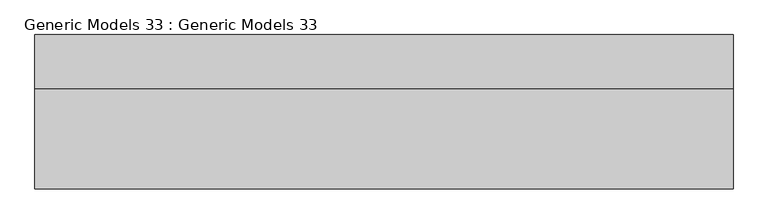
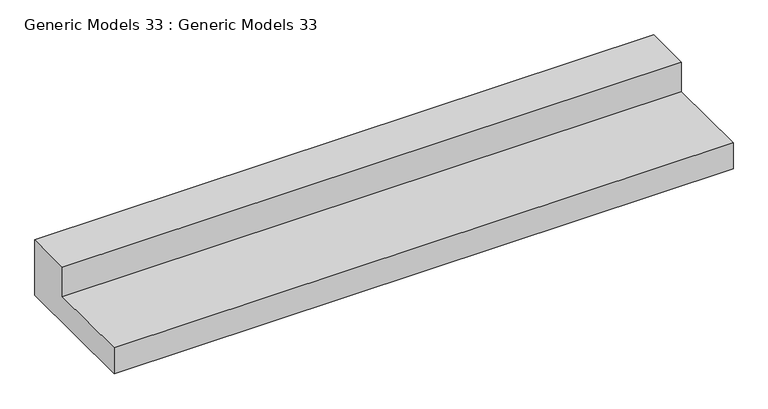
"""IFC4 building model written with IfcOpenShell, lengths in millimetres: proxy geometry, Generic Models 33 : Generic Models 33."""

from ifc_helpers import new_model, si_unit, frame, origin, place, context, project, spatial, polyline, outline, extrude, source, transform, mapped, element, save


def generic_models_33_generic_models_33_1b0ebd61(model_context):
    return source(origin(), model_context, "Body", "SweptSolid", [
        extrude(outline(polyline([(-11268.8679047, 0.0), (-12092.0702746, 0.0), (-12092.0702746, 164.0045243), (-11554.9245764, 164.0045243), (-11554.9245764, 350.0813719), (-11268.8679047, 350.0813719), (-11268.8679047, 0.0)])), frame((-4860.0008859, 0.0, 0.0), z_axis=(1.0, 0.0, 0.0), x_axis=(0.0, 1.0, 0.0)), (0.0, 0.0, 1.0), 3718.1997291),
    ])


if __name__ == "__main__":
    model = new_model("IFC4")
    model_context = context("Model", 3, world=origin())
    ifc_project = project(units=[si_unit("LENGTHUNIT", "METRE", prefix="MILLI")], contexts=[model_context])
    site = spatial("IfcSite", under=ifc_project)
    building = spatial("IfcBuilding", under=site)
    placement = place(None, origin())
    generic_models_33_generic_models_33_shape = generic_models_33_generic_models_33_1b0ebd61(model_context)
    element("IfcBuildingElementProxy", 1, Name="Generic Models 33 : Generic Models 33", ObjectType="Generic Models 33 : Generic Models 33", at=placement, inside=building, context=model_context, shape_type="MappedRepresentation", body=[
        mapped(generic_models_33_generic_models_33_shape, transform((0.0, 0.0, 0.0), x_axis=(1.0, 0.0, 0.0), y_axis=(0.0, 1.0, 0.0), z_axis=(0.0, 0.0, 1.0))),
    ])
    save(model, "model.ifc")

# Revit data of these elements
# Element 1 (IfcBuildingElementProxy, "Generic Models 33 : Generic Models 33")
#   Materials on its faces: "Tile, Porcelain, 4in"
# Materials
#   "Tile, Porcelain, 4in": class "Generic", colour RGB 89 87 158, transparency 0, Description = "Porcelain tile, 4\", white", Cost = 0
